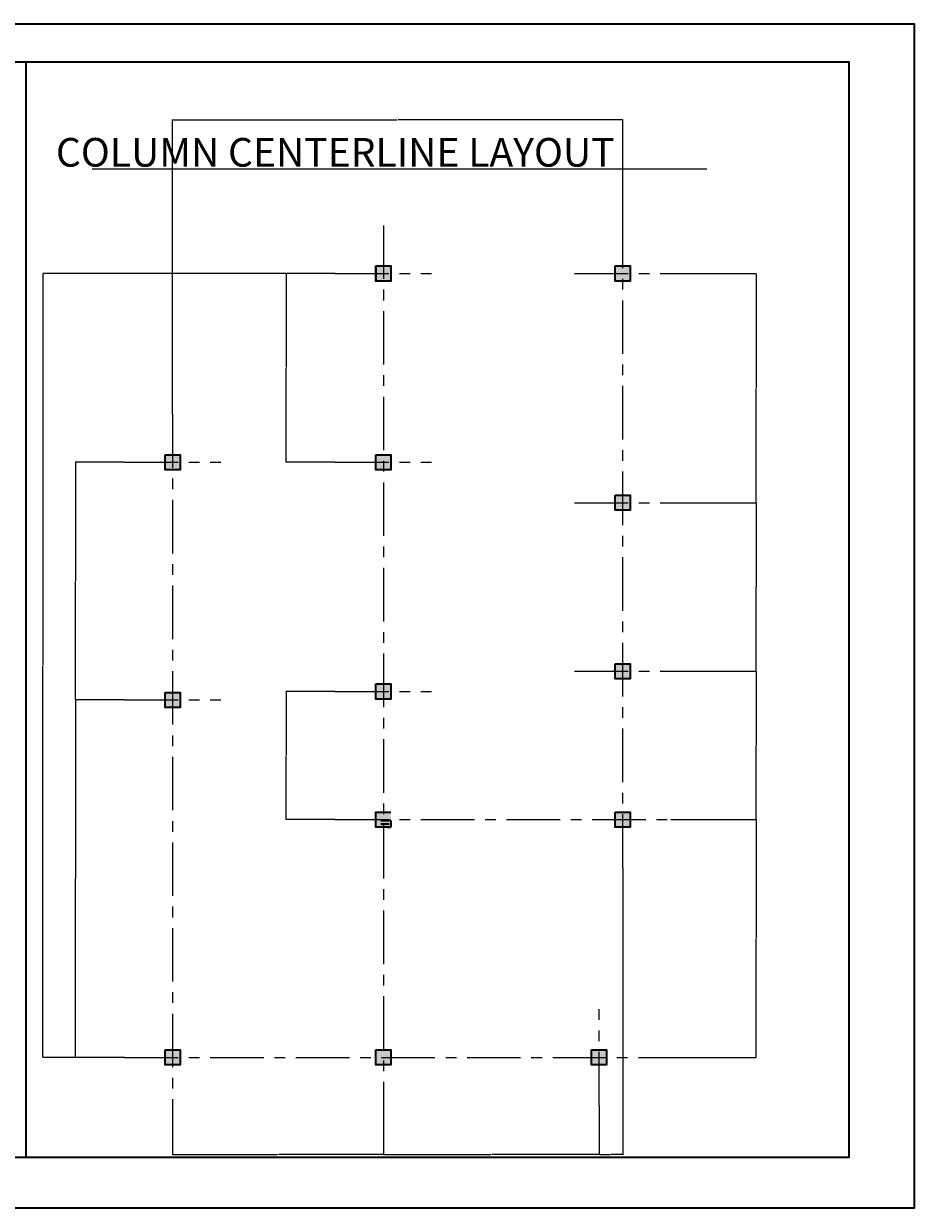
# Model space of a CAD drawing. Units: inches. Extents: x 1762 to 3150, y 1680 to 2382.
# Tile 6 of 6: x 2622 to 3150, y 1680 to 2382. Entities that reach past the tile are written whole.
import ezdxf

# ---------------------------------------------------------------- set-up
doc = ezdxf.new("R2010")
doc.units = ezdxf.units.IN
doc.linetypes.add('CENTER', pattern=[50.8, 31.75, -6.35, 6.35, -6.35])
for name, color, linetype, lineweight in [('A-ANNO-DIMS', 2, 'Continuous', 18), ('A-ANNO-TEXT', 7, 'Continuous', 25), ('A-ANNO-TTLB', 7, 'Continuous', 35), ('S-COLS', 1, 'Continuous', 35), ('S-COLS-PATT', 1, 'Continuous', 13), ('S-GRID', 8, 'CENTER', 13)]:
    doc.layers.add(name, color=color, linetype=linetype, lineweight=lineweight)
doc.styles.get("Standard").update_dxf_attribs({"font": 'arial.ttf'})
doc.dimstyles.get("Standard").update_dxf_attribs({"dimtxt": 0.18, "dimasz": 0.18, "dimexe": 0.18, "dimexo": 0.0625, "dimgap": 0.09, "dimtad": 0, "dimtih": 1, "dimtoh": 1, "dimdec": 4, "dimzin": 0, "dimdsep": 46, "dimtxsty": 'Standard', "dimcen": 0.09, "dimadec": 0, "dimazin": 0, "dimtfac": 1, "dimtdec": 4, "dimtofl": 0, "dimtmove": 0, "dimatfit": 3, "dimfxl": 1, "dimtolj": 1, "dimtzin": 0, "dimarcsym": 0})

# ---------------------------------------------------------------- blocks, each defined once
blk = doc.blocks.new('COL-9X9IN')
h = blk.add_hatch(color=256)
h.dxf.hatch_style = 1
h.paths.add_polyline_path([(0, 0), (9, 0), (9, 9), (0, 9)])
blk.add_lwpolyline([(0, 9), (9, 9), (9, 0), (0, 0)], close=True)
blk = doc.blocks.new('*D82')
at = {"layer": 'A-ANNO-DIMS', "color": 0, "lineweight": -2, "transparency": 16777216}
for p, q in [((2710.28, 1740.57), (2710.28, 1711.35)), ((2835.28, 1740.57), (2835.28, 1711.35)), ((2710.46, 1711.53), (2772.5, 1711.53)), ((2835.1, 1711.53), (2773.06, 1711.53))]:
    blk.add_line(p, q, dxfattribs=at)
at = {"layer": 'A-ANNO-DIMS', "color": 0, "transparency": 16777216}
for points in [[(2710.46, 1711.56), (2710.46, 1711.5), (2710.28, 1711.53)], [(2835.1, 1711.56), (2835.1, 1711.5), (2835.28, 1711.53)]]:
    blk.add_solid(points, dxfattribs=at)
at = {"layer": 'Defpoints', "color": 0, "transparency": 16777216}
for p in [(2710.28, 1740.63), (2835.28, 1740.63), (2835.28, 1711.53)]:
    blk.add_point(p, dxfattribs=at)
at = {"layer": 'A-ANNO-DIMS', "color": 0, "transparency": 16777216, "insert": (2772.78, 1711.53), "char_height": 0.18, "attachment_point": 5}
blk.add_mtext('\\A1;125', dxfattribs=at)
blk = doc.blocks.new('*D83')
at = {"layer": 'A-ANNO-DIMS', "color": 0, "lineweight": -2, "transparency": 16777216}
for p, q in [((2835.28, 1740.57), (2835.28, 1711.35)), ((2963.28, 1740.57), (2963.28, 1711.35)), ((2835.46, 1711.53), (2899, 1711.53)), ((2963.1, 1711.53), (2899.56, 1711.53))]:
    blk.add_line(p, q, dxfattribs=at)
at = {"layer": 'A-ANNO-DIMS', "color": 0, "transparency": 16777216}
for points in [[(2835.46, 1711.56), (2835.46, 1711.5), (2835.28, 1711.53)], [(2963.1, 1711.56), (2963.1, 1711.5), (2963.28, 1711.53)]]:
    blk.add_solid(points, dxfattribs=at)
at = {"layer": 'Defpoints', "color": 0, "transparency": 16777216}
for p in [(2835.28, 1740.63), (2963.28, 1740.63), (2963.28, 1711.53)]:
    blk.add_point(p, dxfattribs=at)
at = {"layer": 'A-ANNO-DIMS', "color": 0, "transparency": 16777216, "insert": (2899.28, 1711.53), "char_height": 0.18, "attachment_point": 5}
blk.add_mtext('\\A1;128', dxfattribs=at)
blk = doc.blocks.new('*D84')
at = {"layer": 'A-ANNO-DIMS', "color": 0, "lineweight": -2, "transparency": 16777216}
for p, q in [((2977.28, 1881.57), (2977.28, 1711.35)), ((2963.28, 1740.57), (2963.28, 1711.35)), ((2963.46, 1711.53), (2970.07, 1711.53)), ((2977.1, 1711.53), (2970.49, 1711.53))]:
    blk.add_line(p, q, dxfattribs=at)
at = {"layer": 'A-ANNO-DIMS', "color": 0, "transparency": 16777216}
for points in [[(2963.46, 1711.56), (2963.46, 1711.5), (2963.28, 1711.53)], [(2977.1, 1711.56), (2977.1, 1711.5), (2977.28, 1711.53)]]:
    blk.add_solid(points, dxfattribs=at)
at = {"layer": 'Defpoints', "color": 0, "transparency": 16777216}
for p in [(2977.28, 1881.63), (2963.28, 1740.63), (2977.28, 1711.53)]:
    blk.add_point(p, dxfattribs=at)
at = {"layer": 'A-ANNO-DIMS', "color": 0, "transparency": 16777216, "insert": (2970.28, 1711.53), "char_height": 0.18, "attachment_point": 5}
blk.add_mtext('\\A1;14', dxfattribs=at)
blk = doc.blocks.new('*D85')
at = {"layer": 'A-ANNO-DIMS', "color": 0, "lineweight": -2, "transparency": 16777216}
for p, q in [((2710.28, 2150.69), (2710.28, 2325.46)), ((2710.46, 2325.28), (2843.49, 2325.28)), ((2977.1, 2325.28), (2844.07, 2325.28)), ((2977.28, 2262.69), (2977.28, 2325.46))]:
    blk.add_line(p, q, dxfattribs=at)
at = {"layer": 'A-ANNO-DIMS', "color": 0, "transparency": 16777216}
for points in [[(2710.46, 2325.31), (2710.46, 2325.25), (2710.28, 2325.28)], [(2977.1, 2325.31), (2977.1, 2325.25), (2977.28, 2325.28)]]:
    blk.add_solid(points, dxfattribs=at)
at = {"layer": 'Defpoints', "color": 0, "transparency": 16777216}
for p in [(2977.28, 2325.28), (2977.28, 2262.63), (2710.28, 2150.63)]:
    blk.add_point(p, dxfattribs=at)
at = {"layer": 'A-ANNO-DIMS', "color": 0, "transparency": 16777216, "insert": (2843.78, 2325.28), "char_height": 0.18, "attachment_point": 5}
blk.add_mtext('\\A1;267', dxfattribs=at)
blk = doc.blocks.new('*D86')
at = {"layer": 'A-ANNO-DIMS', "color": 0, "lineweight": -2, "transparency": 16777216}
for p, q in [((2806.72, 2234.13), (2633.17, 2234.13)), ((2633.35, 2233.95), (2633.35, 2001.81)), ((2633.35, 1769.31), (2633.35, 2001.45)), ((2681.72, 1769.13), (2633.17, 1769.13))]:
    blk.add_line(p, q, dxfattribs=at)
at = {"layer": 'A-ANNO-DIMS', "color": 0, "transparency": 16777216}
for points in [[(2633.32, 2233.95), (2633.38, 2233.95), (2633.35, 2234.13)], [(2633.32, 1769.31), (2633.38, 1769.31), (2633.35, 1769.13)]]:
    blk.add_solid(points, dxfattribs=at)
at = {"layer": 'Defpoints', "color": 0, "transparency": 16777216}
for p in [(2633.35, 2234.13), (2806.78, 2234.13), (2681.78, 1769.13)]:
    blk.add_point(p, dxfattribs=at)
at = {"layer": 'A-ANNO-DIMS', "color": 0, "transparency": 16777216, "insert": (2633.35, 2001.63), "char_height": 0.18, "attachment_point": 5}
blk.add_mtext('\\A1;465', dxfattribs=at)
blk = doc.blocks.new('*D87')
at = {"layer": 'A-ANNO-DIMS', "color": 0, "lineweight": -2, "transparency": 16777216}
for p, q in [((2681.72, 1981.13), (2652.5, 1981.13)), ((2652.68, 1980.95), (2652.68, 1875.31)), ((2652.68, 1769.31), (2652.68, 1874.95)), ((2681.72, 1769.13), (2652.5, 1769.13))]:
    blk.add_line(p, q, dxfattribs=at)
at = {"layer": 'A-ANNO-DIMS', "color": 0, "transparency": 16777216}
for points in [[(2652.65, 1980.95), (2652.71, 1980.95), (2652.68, 1981.13)], [(2652.65, 1769.31), (2652.71, 1769.31), (2652.68, 1769.13)]]:
    blk.add_solid(points, dxfattribs=at)
at = {"layer": 'Defpoints', "color": 0, "transparency": 16777216}
for p in [(2652.68, 1981.13), (2681.78, 1981.13), (2681.78, 1769.13)]:
    blk.add_point(p, dxfattribs=at)
at = {"layer": 'A-ANNO-DIMS', "color": 0, "transparency": 16777216, "insert": (2652.68, 1875.13), "char_height": 0.18, "attachment_point": 5}
blk.add_mtext('\\A1;212', dxfattribs=at)
blk = doc.blocks.new('*D88')
at = {"layer": 'A-ANNO-DIMS', "color": 0, "lineweight": -2, "transparency": 16777216}
for p, q in [((2681.72, 2122.13), (2652.5, 2122.13)), ((2652.68, 2121.95), (2652.68, 2051.81)), ((2652.68, 1981.31), (2652.68, 2051.45)), ((2681.72, 1981.13), (2652.5, 1981.13))]:
    blk.add_line(p, q, dxfattribs=at)
at = {"layer": 'A-ANNO-DIMS', "color": 0, "transparency": 16777216}
for points in [[(2652.65, 2121.95), (2652.71, 2121.95), (2652.68, 2122.13)], [(2652.65, 1981.31), (2652.71, 1981.31), (2652.68, 1981.13)]]:
    blk.add_solid(points, dxfattribs=at)
at = {"layer": 'Defpoints', "color": 0, "transparency": 16777216}
for p in [(2652.68, 2122.13), (2681.78, 2122.13), (2681.78, 1981.13)]:
    blk.add_point(p, dxfattribs=at)
at = {"layer": 'A-ANNO-DIMS', "color": 0, "transparency": 16777216, "insert": (2652.68, 2051.63), "char_height": 0.18, "attachment_point": 5}
blk.add_mtext('\\A1;141', dxfattribs=at)
blk = doc.blocks.new('*D89')
at = {"layer": 'A-ANNO-DIMS', "color": 0, "lineweight": -2, "transparency": 16777216}
for p, q in [((2806.72, 2234.13), (2777.5, 2234.13)), ((2777.68, 2233.95), (2777.68, 2178.31)), ((2777.68, 2122.31), (2777.68, 2177.95)), ((2806.72, 2122.13), (2777.5, 2122.13))]:
    blk.add_line(p, q, dxfattribs=at)
at = {"layer": 'A-ANNO-DIMS', "color": 0, "transparency": 16777216}
for points in [[(2777.65, 2233.95), (2777.71, 2233.95), (2777.68, 2234.13)], [(2777.65, 2122.31), (2777.71, 2122.31), (2777.68, 2122.13)]]:
    blk.add_solid(points, dxfattribs=at)
at = {"layer": 'Defpoints', "color": 0, "transparency": 16777216}
for p in [(2777.68, 2234.13), (2806.78, 2234.13), (2806.78, 2122.13)]:
    blk.add_point(p, dxfattribs=at)
at = {"layer": 'A-ANNO-DIMS', "color": 0, "transparency": 16777216, "insert": (2777.68, 2178.13), "char_height": 0.18, "attachment_point": 5}
blk.add_mtext('\\A1;112', dxfattribs=at)
blk = doc.blocks.new('*D90')
at = {"layer": 'A-ANNO-DIMS', "color": 0, "lineweight": -2, "transparency": 16777216}
for p, q in [((3005.84, 1910.13), (3056.58, 1910.13)), ((3056.4, 1909.95), (3056.4, 1839.81)), ((3056.4, 1769.31), (3056.4, 1839.45)), ((2991.84, 1769.13), (3056.58, 1769.13))]:
    blk.add_line(p, q, dxfattribs=at)
at = {"layer": 'A-ANNO-DIMS', "color": 0, "transparency": 16777216}
for points in [[(3056.37, 1909.95), (3056.43, 1909.95), (3056.4, 1910.13)], [(3056.37, 1769.31), (3056.43, 1769.31), (3056.4, 1769.13)]]:
    blk.add_solid(points, dxfattribs=at)
at = {"layer": 'Defpoints', "color": 0, "transparency": 16777216}
for p in [(3005.78, 1910.13), (3056.4, 1910.13), (2991.78, 1769.13)]:
    blk.add_point(p, dxfattribs=at)
at = {"layer": 'A-ANNO-DIMS', "color": 0, "transparency": 16777216, "insert": (3056.4, 1839.63), "char_height": 0.18, "attachment_point": 5}
blk.add_mtext('\\A1;141', dxfattribs=at)
blk = doc.blocks.new('*D91')
at = {"layer": 'A-ANNO-DIMS', "color": 0, "lineweight": -2, "transparency": 16777216}
for p, q in [((3005.84, 1998.13), (3056.58, 1998.13)), ((3056.4, 1997.95), (3056.4, 1954.31)), ((3056.4, 1910.31), (3056.4, 1953.95)), ((3005.84, 1910.13), (3056.58, 1910.13))]:
    blk.add_line(p, q, dxfattribs=at)
at = {"layer": 'A-ANNO-DIMS', "color": 0, "transparency": 16777216}
for points in [[(3056.37, 1997.95), (3056.43, 1997.95), (3056.4, 1998.13)], [(3056.37, 1910.31), (3056.43, 1910.31), (3056.4, 1910.13)]]:
    blk.add_solid(points, dxfattribs=at)
at = {"layer": 'Defpoints', "color": 0, "transparency": 16777216}
for p in [(3005.78, 1998.13), (3056.4, 1998.13), (3005.78, 1910.13)]:
    blk.add_point(p, dxfattribs=at)
at = {"layer": 'A-ANNO-DIMS', "color": 0, "transparency": 16777216, "insert": (3056.4, 1954.13), "char_height": 0.18, "attachment_point": 5}
blk.add_mtext('\\A1;88', dxfattribs=at)
blk = doc.blocks.new('*D92')
at = {"layer": 'A-ANNO-DIMS', "color": 0, "lineweight": -2, "transparency": 16777216}
for p, q in [((3005.84, 2098.13), (3056.58, 2098.13)), ((3056.4, 2097.95), (3056.4, 2048.31)), ((3056.4, 1998.31), (3056.4, 2047.95)), ((3005.84, 1998.13), (3056.58, 1998.13))]:
    blk.add_line(p, q, dxfattribs=at)
at = {"layer": 'A-ANNO-DIMS', "color": 0, "transparency": 16777216}
for points in [[(3056.37, 2097.95), (3056.43, 2097.95), (3056.4, 2098.13)], [(3056.37, 1998.31), (3056.43, 1998.31), (3056.4, 1998.13)]]:
    blk.add_solid(points, dxfattribs=at)
at = {"layer": 'Defpoints', "color": 0, "transparency": 16777216}
for p in [(3005.78, 2098.13), (3056.4, 2098.13), (3005.78, 1998.13)]:
    blk.add_point(p, dxfattribs=at)
at = {"layer": 'A-ANNO-DIMS', "color": 0, "transparency": 16777216, "insert": (3056.4, 2048.13), "char_height": 0.18, "attachment_point": 5}
blk.add_mtext('\\A1;100', dxfattribs=at)
blk = doc.blocks.new('*D93')
at = {"layer": 'A-ANNO-DIMS', "color": 0, "lineweight": -2, "transparency": 16777216}
for p, q in [((3005.84, 2234.13), (3056.58, 2234.13)), ((3056.4, 2233.95), (3056.4, 2166.31)), ((3056.4, 2098.31), (3056.4, 2165.95)), ((3005.84, 2098.13), (3056.58, 2098.13))]:
    blk.add_line(p, q, dxfattribs=at)
at = {"layer": 'A-ANNO-DIMS', "color": 0, "transparency": 16777216}
for points in [[(3056.37, 2233.95), (3056.43, 2233.95), (3056.4, 2234.13)], [(3056.37, 2098.31), (3056.43, 2098.31), (3056.4, 2098.13)]]:
    blk.add_solid(points, dxfattribs=at)
at = {"layer": 'Defpoints', "color": 0, "transparency": 16777216}
for p in [(3005.78, 2234.13), (3056.4, 2234.13), (3005.78, 2098.13)]:
    blk.add_point(p, dxfattribs=at)
at = {"layer": 'A-ANNO-DIMS', "color": 0, "transparency": 16777216, "insert": (3056.4, 2166.13), "char_height": 0.18, "attachment_point": 5}
blk.add_mtext('\\A1;136', dxfattribs=at)
blk = doc.blocks.new('*D94')
at = {"layer": 'A-ANNO-DIMS', "color": 0, "lineweight": -2, "transparency": 16777216}
for p, q in [((2806.72, 1986.13), (2777.5, 1986.13)), ((2777.68, 1985.95), (2777.68, 1948.31)), ((2777.68, 1910.31), (2777.68, 1947.95)), ((2806.72, 1910.13), (2777.5, 1910.13))]:
    blk.add_line(p, q, dxfattribs=at)
at = {"layer": 'A-ANNO-DIMS', "color": 0, "transparency": 16777216}
for points in [[(2777.65, 1985.95), (2777.71, 1985.95), (2777.68, 1986.13)], [(2777.65, 1910.31), (2777.71, 1910.31), (2777.68, 1910.13)]]:
    blk.add_solid(points, dxfattribs=at)
at = {"layer": 'Defpoints', "color": 0, "transparency": 16777216}
for p in [(2777.68, 1986.13), (2806.78, 1986.13), (2806.78, 1910.13)]:
    blk.add_point(p, dxfattribs=at)
at = {"layer": 'A-ANNO-DIMS', "color": 0, "transparency": 16777216, "insert": (2777.68, 1948.13), "char_height": 0.18, "attachment_point": 5}
blk.add_mtext('\\A1;76', dxfattribs=at)

msp = doc.modelspace()

# ---------------------------------------------------------------- hatches: boundary and pattern name
at = {"layer": 'S-COLS-PATT'}
h = msp.add_hatch(color=256, dxfattribs=at)
h.dxf.hatch_style = 1
h.paths.add_polyline_path([(2830.7796, 1905.6284), (2839.7796, 1905.6284), (2839.7796, 1914.6284), (2830.7796, 1914.6284)])

# ---------------------------------------------------------------- linework, layer by layer
at = {"layer": 'A-ANNO-TEXT'}
msp.add_line((2662.4489, 2296.1803), (3027.2992, 2296.1803), dxfattribs=at)
at = {"layer": 'A-ANNO-TTLB'}
msp.add_line((2623.1666, 2359.5805), (2623.1666, 1709.6712), dxfattribs=at)
for points in [[(1762.4998, 2382.3025), (3150.3176, 2382.3025), (3150.3176, 1679.5742), (1762.4998, 1679.5742)], [(1799.0337, 2359.5805), (3111.4319, 2359.5805), (3111.4319, 1709.6712), (1799.0337, 1709.6712)]]:
    msp.add_lwpolyline(points, close=True, dxfattribs=at)
at = {"layer": 'S-COLS'}
for p, q in [((2830.7796, 2238.6284), (2830.7796, 2229.6284)), ((2833.7796, 1909.6284), (2838.7796, 1909.6284)), ((2839.7796, 1909.6284), (2833.7796, 1909.6284)), ((2833.7796, 1907.6284), (2838.7796, 1907.6284)), ((2837.7796, 1905.6284), (2839.7796, 1905.6284)), ((2839.7796, 1909.6284), (2839.7796, 1905.6284)), ((2830.7796, 1773.6284), (2832.7796, 1773.6284))]:
    msp.add_line(p, q, dxfattribs=at)
msp.add_lwpolyline([(2839.7796, 1905.6284), (2830.7796, 1905.6284), (2830.7796, 1914.6284), (2839.7796, 1914.6284)], dxfattribs=at)
at = {"layer": 'S-GRID'}
for p, q in [((2835.2796, 2262.6284), (2835.2796, 1740.6284)), ((2977.2796, 1881.6284), (2977.2796, 2262.6284)), ((2806.7796, 2234.1284), (2863.7796, 2234.1284)), ((2948.7796, 2234.1284), (3005.7796, 2234.1284)), ((2710.2796, 2150.6284), (2710.2796, 1740.6284)), ((2681.7796, 2122.1284), (2738.7796, 2122.1284)), ((2806.7796, 2122.1284), (2863.7796, 2122.1284)), ((2948.7796, 2098.1284), (3005.7796, 2098.1284)), ((2948.7796, 1998.1284), (3005.7796, 1998.1284)), ((2806.7796, 1986.1284), (2863.7796, 1986.1284)), ((2681.7796, 1981.1284), (2738.7796, 1981.1284)), ((2806.7796, 1910.1284), (3005.7796, 1910.1284)), ((2963.2796, 1740.6284), (2963.2796, 1797.6284)), ((2681.7796, 1769.1284), (2991.7796, 1769.1284))]:
    msp.add_line(p, q, dxfattribs=at)

# ---------------------------------------------------------------- block references
at = {"layer": 'S-COLS'}
for p in [(2830.78, 2229.628), (2972.78, 2229.628), (2705.78, 2117.628), (2830.78, 2117.628), (2972.78, 2093.628), (2972.78, 1993.628), (2830.78, 1981.628), (2705.78, 1976.628), (2972.78, 1905.628), (2705.78, 1764.628), (2830.78, 1764.628), (2958.78, 1764.628)]:
    msp.add_blockref('COL-9X9IN', p, dxfattribs=at)

# ---------------------------------------------------------------- texts
at = {"layer": 'A-ANNO-TEXT'}
msp.add_text('               COLUMN CENTERLINE LAYOUT', height=17, dxfattribs=at).set_placement((2563.0864, 2297.5007))

# ---------------------------------------------------------------- dimensions: what is measured, and where the dimension line sits
at = {"layer": 'A-ANNO-DIMS'}
for base, p1, p2, picture, middle in [((2977.2796, 2325.2803), (2710.2796, 2150.6284), (2977.2796, 2262.6284), '*D85', (2843.7796, 2325.2803)), ((2977.2796, 1711.5284), (2963.2796, 1740.6284), (2977.2796, 1881.6284), '*D84', (2970.2796, 1711.5284)), ((2835.2796, 1711.5284), (2710.2796, 1740.6284), (2835.2796, 1740.6284), '*D82', (2772.7796, 1711.5284)), ((2963.2796, 1711.5284), (2835.2796, 1740.6284), (2963.2796, 1740.6284), '*D83', (2899.2796, 1711.5284))]:
    dim = msp.add_linear_dim(base=base, p1=p1, p2=p2, dimstyle='Standard', override={"dimdec": 0, "dimlfac": 1, "dimrnd": 0, "dimzin": 0, "dimdsep": 46, "dimlunit": 2}, dxfattribs=at)
    dim.commit()
    dim.dimension.update_dxf_attribs({"geometry": picture, "text_midpoint": middle})
for base, p1, p2, picture, middle in [((2633.3489, 2234.1284), (2681.7796, 1769.1284), (2806.7796, 2234.1284), '*D86', (2633.3489, 2001.6284)), ((2777.6796, 2234.1284), (2806.7796, 2122.1284), (2806.7796, 2234.1284), '*D89', (2777.6796, 2178.1284)), ((3056.3992, 2234.1284), (3005.7796, 2098.1284), (3005.7796, 2234.1284), '*D93', (3056.3992, 2166.1284)), ((2652.6796, 2122.1284), (2681.7796, 1981.1284), (2681.7796, 2122.1284), '*D88', (2652.6796, 2051.6284)), ((3056.3992, 2098.1284), (3005.7796, 1998.1284), (3005.7796, 2098.1284), '*D92', (3056.3992, 2048.1284)), ((3056.3992, 1998.1284), (3005.7796, 1910.1284), (3005.7796, 1998.1284), '*D91', (3056.3992, 1954.1284)), ((2777.6796, 1986.1284), (2806.7796, 1910.1284), (2806.7796, 1986.1284), '*D94', (2777.6796, 1948.1284)), ((2652.6796, 1981.1284), (2681.7796, 1769.1284), (2681.7796, 1981.1284), '*D87', (2652.6796, 1875.1284)), ((3056.3992, 1910.1284), (2991.7796, 1769.1284), (3005.7796, 1910.1284), '*D90', (3056.3992, 1839.6284))]:
    dim = msp.add_linear_dim(base=base, p1=p1, p2=p2, angle=90, dimstyle='Standard', override={"dimdec": 0, "dimlfac": 1, "dimrnd": 0, "dimzin": 0, "dimdsep": 46, "dimlunit": 2}, dxfattribs=at)
    dim.commit()
    dim.dimension.update_dxf_attribs({"geometry": picture, "text_midpoint": middle})

doc.saveas('drawing.dxf')
